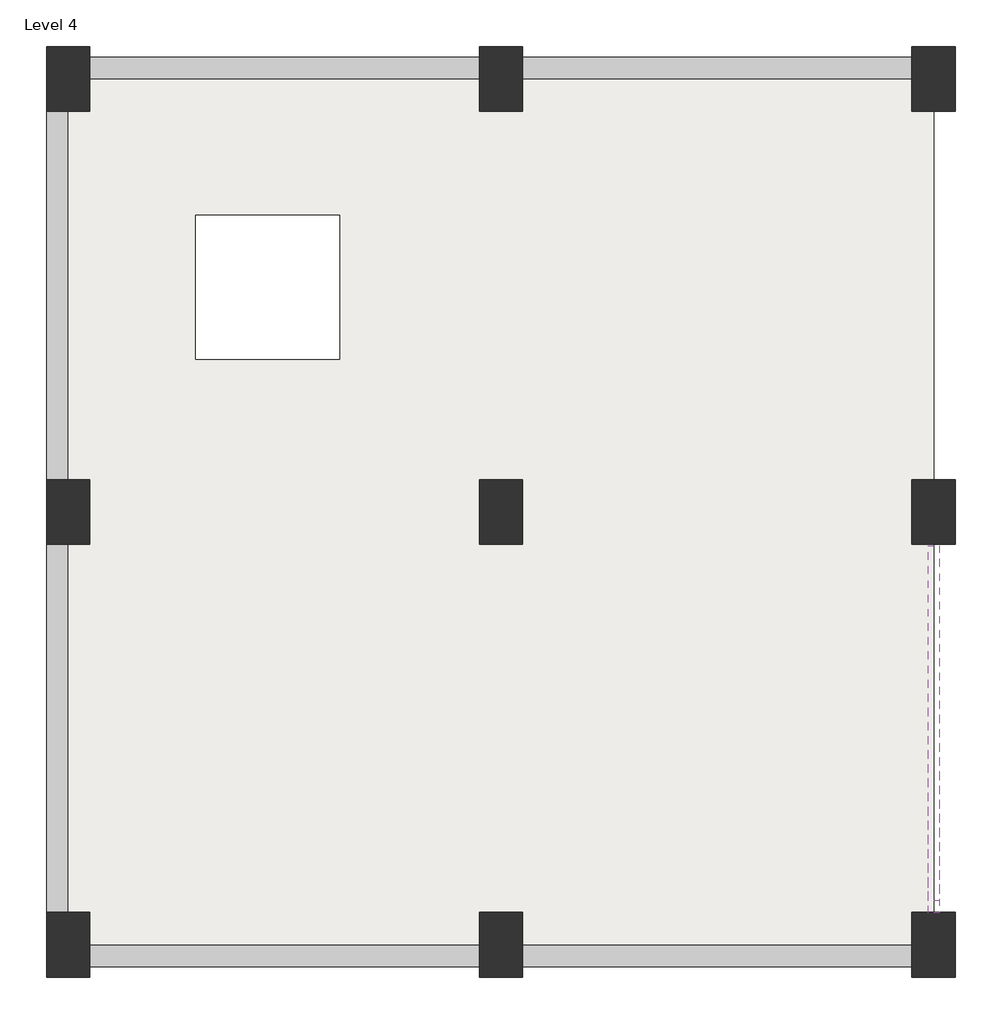
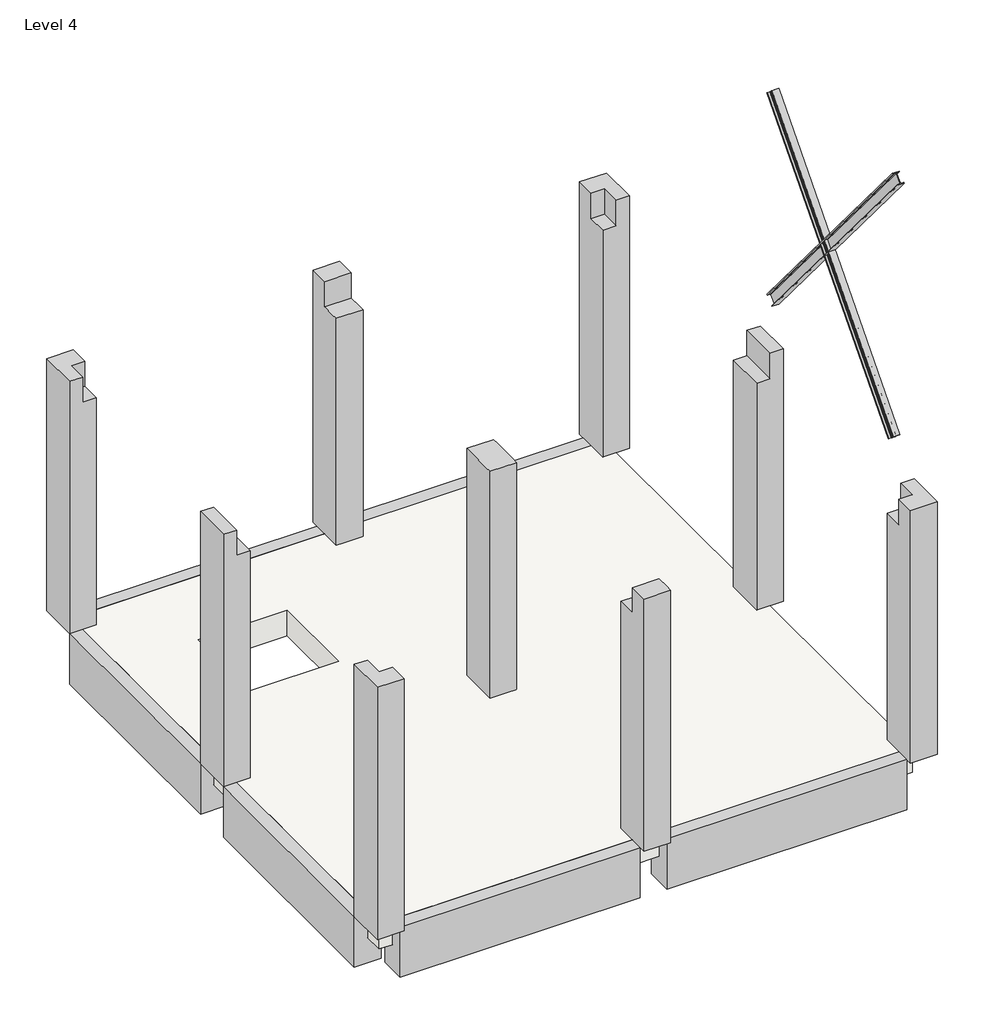
# One storey: 9 columns, 4 beams, 2 members, 2 slabs.
"""IFC4 building model written with IfcOpenShell, lengths in millimetres."""

from ifc_helpers import new_model, si_unit, frame, origin, place, context, project, spatial, polyline, outline, extrude, faceted_brep, transform, mapped, element, save
from components import ub_universal_beams_ub127x76x13_5289bed7, ub_universal_beams_ub127x76x13_b97c8348

model = new_model("IFC4")

# Units and contexts
model_context = context("Model", 3, world=origin())
ifc_project = project(units=[si_unit("LENGTHUNIT", "METRE", prefix="MILLI")], contexts=[model_context])

# Site, building, storey
site = spatial("IfcSite", under=ifc_project)
building = spatial("IfcBuilding", under=site)
storey = spatial("IfcBuildingStorey", under=building, Name="Level 4", Elevation=9000.0)

# Beams
placement = place(None, origin())
element("IfcBeam", 1, ObjectType="Concrete-Rectangular Beam : 300 x 600mm", at=placement, inside=storey, context=model_context, shape_type="SweptSolid", body=[
    extrude(outline(polyline([(526.3372902, 8400.0), (226.3372902, 8400.0), (226.3372902, 8700.0), (376.3372902, 8700.0), (376.3372902, 9000.0), (526.3372902, 9000.0), (526.3372902, 8400.0)])), frame((2068.7595868, 0.0, 0.0), z_axis=(1.0, 0.0, 0.0), x_axis=(0.0, 1.0, 0.0)), (0.0, 0.0, 1.0), 2700.0),
    extrude(outline(polyline([(526.3372902, 8400.0), (226.3372902, 8400.0), (226.3372902, 8700.0), (376.3372902, 8700.0), (376.3372902, 9000.0), (526.3372902, 9000.0), (526.3372902, 8400.0)])), frame((-931.2404132, 0.0, 0.0), z_axis=(1.0, 0.0, 0.0), x_axis=(0.0, 1.0, 0.0)), (0.0, 0.0, 1.0), 2700.0),
])
element("IfcBeam", 2, ObjectType="Concrete-Rectangular Beam : 300 x 600mm", at=placement, inside=storey, context=model_context, shape_type="SweptSolid", body=[
    extrude(outline(polyline([(-5773.6627098, 8400.0), (-5773.6627098, 9000.0), (-5623.6627098, 9000.0), (-5623.6627098, 8700.0), (-5473.6627098, 8700.0), (-5473.6627098, 8400.0), (-5773.6627098, 8400.0)])), frame((2068.7595868, 0.0, 0.0), z_axis=(1.0, 0.0, 0.0), x_axis=(0.0, 1.0, 0.0)), (0.0, 0.0, 1.0), 2700.0),
    extrude(outline(polyline([(-5773.6627098, 8400.0), (-5773.6627098, 9000.0), (-5623.6627098, 9000.0), (-5623.6627098, 8700.0), (-5473.6627098, 8700.0), (-5473.6627098, 8400.0), (-5773.6627098, 8400.0)])), frame((-931.2404132, 0.0, 0.0), z_axis=(1.0, 0.0, 0.0), x_axis=(0.0, 1.0, 0.0)), (0.0, 0.0, 1.0), 2700.0),
])
element("IfcBeam", 3, ObjectType="Concrete-Rectangular Beam : 300 x 600mm", at=placement, inside=storey, context=model_context, shape_type="SweptSolid", body=[
    extrude(outline(polyline([(9000.0, -1231.2404132), (8400.0, -1231.2404132), (8400.0, -931.2404132), (8700.0, -931.2404132), (8700.0, -1081.2404132), (9000.0, -1081.2404132), (9000.0, -1231.2404132)])), frame((0.0, -5398.6627098, 0.0), z_axis=(0.0, 1.0, 0.0), x_axis=(0.0, 0.0, 1.0)), (0.0, 0.0, 1.0), 2550.0),
    extrude(outline(polyline([(9000.0, -1231.2404132), (8400.0, -1231.2404132), (8400.0, -931.2404132), (8700.0, -931.2404132), (8700.0, -1081.2404132), (9000.0, -1081.2404132), (9000.0, -1231.2404132)])), frame((0.0, -2398.6627098, 0.0), z_axis=(0.0, 1.0, 0.0), x_axis=(0.0, 0.0, 1.0)), (0.0, 0.0, 1.0), 2550.0),
])
element("IfcBeam", 4, ObjectType="Concrete-Rectangular Beam : 300 x 600mm", at=placement, inside=storey, context=model_context, shape_type="SweptSolid", body=[
    extrude(outline(polyline([(2068.7595868, -2773.6627098), (2068.7595868, -2473.6627098), (4768.7595868, -2473.6627098), (4768.7595868, -2773.6627098), (2068.7595868, -2773.6627098)])), frame((0.0, 0.0, 8400.0), z_axis=(0.0, 0.0, 1.0), x_axis=(1.0, 0.0, 0.0)), (0.0, 0.0, 1.0), 300.0),
    extrude(outline(polyline([(-931.2404132, -2773.6627098), (-931.2404132, -2473.6627098), (1768.7595868, -2473.6627098), (1768.7595868, -2773.6627098), (-931.2404132, -2773.6627098)])), frame((0.0, 0.0, 8400.0), z_axis=(0.0, 0.0, 1.0), x_axis=(1.0, 0.0, 0.0)), (0.0, 0.0, 1.0), 300.0),
])

# Columns
element("IfcColumn", 5, ObjectType="Concrete-Rectangular-Column : 300 x 450mm", at=placement, inside=storey, context=model_context, shape_type="Brep", body=[
    faceted_brep([(-1231.2404132, -5848.6627098, 12000.0), (-931.2404132, -5848.6627098, 12000.0), (-931.2404132, -5623.6627098, 12000.0), (-1081.2404132, -5623.6627098, 12000.0), (-1081.2404132, -5398.6627098, 12000.0), (-1231.2404132, -5398.6627098, 12000.0), (-1231.2404132, -5848.6627098, 9000.0), (-1231.2404132, -5398.6627098, 9000.0), (-931.2404132, -5398.6627098, 9000.0), (-931.2404132, -5848.6627098, 9000.0), (-931.2404132, -5398.6627098, 11700.0), (-931.2404132, -5623.6627098, 11700.0), (-1081.2404132, -5398.6627098, 11700.0), (-1081.2404132, -5623.6627098, 11700.0)], [[[0, 1, 2, 3, 4, 5]], [[6, 7, 8, 9]], [[1, 0, 6, 9]], [[9, 8, 10, 11, 2, 1]], [[8, 7, 5, 4, 12, 10]], [[0, 5, 7, 6]], [[12, 13, 11, 10]], [[13, 3, 2, 11]], [[3, 13, 12, 4]]]),
])
element("IfcColumn", 6, ObjectType="Concrete-Rectangular-Column : 300 x 450mm", at=placement, inside=storey, context=model_context, shape_type="Brep", body=[
    faceted_brep([(1768.7595868, -5848.6627098, 12000.0), (2068.7595868, -5848.6627098, 12000.0), (2068.7595868, -5773.6627098, 12000.0), (2068.7595868, -5623.6627098, 12000.0), (1768.7595868, -5623.6627098, 12000.0), (1768.7595868, -5773.6627098, 12000.0), (1768.7595868, -5848.6627098, 9000.0), (1768.7595868, -5398.6627098, 9000.0), (2068.7595868, -5398.6627098, 9000.0), (2068.7595868, -5848.6627098, 9000.0), (2068.7595868, -5398.6627098, 11700.0), (2068.7595868, -5473.6627098, 11700.0), (2068.7595868, -5623.6627098, 11700.0), (1768.7595868, -5398.6627098, 11700.0), (1768.7595868, -5623.6627098, 11700.0), (1768.7595868, -5473.6627098, 11700.0)], [[[0, 1, 2, 3, 4, 5]], [[6, 7, 8, 9]], [[1, 0, 6, 9]], [[9, 8, 10, 11, 12, 3, 2, 1]], [[8, 7, 13, 10]], [[7, 6, 0, 5, 4, 14, 15, 13]], [[14, 12, 11, 10, 13, 15]], [[12, 14, 4, 3]]]),
])
element("IfcColumn", 7, ObjectType="Concrete-Rectangular-Column : 300 x 450mm", at=placement, inside=storey, context=model_context, shape_type="Brep", body=[
    faceted_brep([(4768.7595868, -5848.6627098, 12000.0), (5068.7595868, -5848.6627098, 12000.0), (5068.7595868, -5398.6627098, 12000.0), (4918.7595868, -5398.6627098, 12000.0), (4918.7595868, -5623.6627098, 12000.0), (4768.7595868, -5623.6627098, 12000.0), (4768.7595868, -5848.6627098, 9000.0), (4768.7595868, -5398.6627098, 9000.0), (5068.7595868, -5398.6627098, 9000.0), (5068.7595868, -5848.6627098, 9000.0), (4768.7595868, -5398.6627098, 11700.0), (4918.7595868, -5398.6627098, 11700.0), (4768.7595868, -5623.6627098, 11700.0), (4918.7595868, -5623.6627098, 11700.0)], [[[0, 1, 2, 3, 4, 5]], [[6, 7, 8, 9]], [[1, 0, 6, 9]], [[2, 1, 9, 8]], [[8, 7, 10, 11, 3, 2]], [[7, 6, 0, 5, 12, 10]], [[12, 13, 11, 10]], [[13, 4, 3, 11]], [[4, 13, 12, 5]]]),
])
element("IfcColumn", 8, ObjectType="Concrete-Rectangular-Column : 300 x 450mm", at=placement, inside=storey, context=model_context, shape_type="Brep", body=[
    faceted_brep([(-1231.2404132, -2398.6627098, 12000.0), (-1231.2404132, -2848.6627098, 12000.0), (-1081.2404132, -2848.6627098, 12000.0), (-1081.2404132, -2398.6627098, 12000.0), (-1231.2404132, -2848.6627098, 9000.0), (-1231.2404132, -2398.6627098, 9000.0), (-931.2404132, -2398.6627098, 9000.0), (-931.2404132, -2848.6627098, 9000.0), (-931.2404132, -2848.6627098, 11400.0), (-931.2404132, -2848.6627098, 11700.0), (-1081.2404132, -2848.6627098, 11700.0), (-1231.2404132, -2848.6627098, 11400.0), (-931.2404132, -2398.6627098, 11400.0), (-931.2404132, -2398.6627098, 11700.0), (-1231.2404132, -2398.6627098, 11400.0), (-1081.2404132, -2398.6627098, 11700.0)], [[[0, 1, 2, 3]], [[4, 5, 6, 7]], [[4, 7, 8, 9, 10, 2, 1, 11]], [[7, 6, 12, 13, 9, 8]], [[6, 5, 14, 0, 3, 15, 13, 12]], [[1, 0, 14, 5, 4, 11]], [[15, 10, 9, 13]], [[10, 15, 3, 2]]]),
])
element("IfcColumn", 9, ObjectType="Concrete-Rectangular-Column : 300 x 450mm", at=placement, inside=storey, context=model_context, shape_type="Brep", body=[
    faceted_brep([(1768.7595868, -2848.6627098, 9000.0), (1768.7595868, -2398.6627098, 9000.0), (2068.7595868, -2398.6627098, 9000.0), (2068.7595868, -2848.6627098, 9000.0), (2068.7595868, -2848.6627098, 11400.0), (2068.7595868, -2848.6627098, 11700.0), (1768.7595868, -2848.6627098, 11700.0), (1768.7595868, -2848.6627098, 11400.0), (2068.7595868, -2398.6627098, 11400.0), (2068.7595868, -2398.6627098, 11700.0), (2068.7595868, -2473.6627098, 11700.0), (2068.7595868, -2773.6627098, 11700.0), (1768.7595868, -2398.6627098, 11400.0), (1768.7595868, -2398.6627098, 11700.0), (1768.7595868, -2773.6627098, 11700.0), (1768.7595868, -2473.6627098, 11700.0)], [[[0, 1, 2, 3]], [[0, 3, 4, 5, 6, 7]], [[3, 2, 8, 9, 10, 11, 5, 4]], [[2, 1, 12, 13, 9, 8]], [[1, 0, 7, 6, 14, 15, 13, 12]], [[6, 5, 11, 10, 9, 13, 15, 14]]]),
])
element("IfcColumn", 10, ObjectType="Concrete-Rectangular-Column : 300 x 450mm", at=placement, inside=storey, context=model_context, shape_type="Brep", body=[
    faceted_brep([(5068.7595868, -2848.6627098, 12000.0), (5068.7595868, -2398.6627098, 12000.0), (4918.7595868, -2398.6627098, 12000.0), (4918.7595868, -2848.6627098, 12000.0), (4768.7595868, -2848.6627098, 9000.0), (4768.7595868, -2398.6627098, 9000.0), (5068.7595868, -2398.6627098, 9000.0), (5068.7595868, -2848.6627098, 9000.0), (5068.7595868, -2848.6627098, 11400.0), (4918.7595868, -2848.6627098, 11700.0), (4768.7595868, -2848.6627098, 11700.0), (4768.7595868, -2848.6627098, 11400.0), (5068.7595868, -2398.6627098, 11400.0), (4768.7595868, -2398.6627098, 11400.0), (4768.7595868, -2398.6627098, 11700.0), (4918.7595868, -2398.6627098, 11700.0)], [[[0, 1, 2, 3]], [[4, 5, 6, 7]], [[4, 7, 8, 0, 3, 9, 10, 11]], [[1, 0, 8, 7, 6, 12]], [[6, 5, 13, 14, 15, 2, 1, 12]], [[5, 4, 11, 10, 14, 13]], [[9, 15, 14, 10]], [[15, 9, 3, 2]]]),
])
element("IfcColumn", 11, ObjectType="Concrete-Rectangular-Column : 300 x 450mm", at=placement, inside=storey, context=model_context, shape_type="Brep", body=[
    faceted_brep([(-931.2404132, 601.3372902, 12000.0), (-1231.2404132, 601.3372902, 12000.0), (-1231.2404132, 151.3372902, 12000.0), (-1081.2404132, 151.3372902, 12000.0), (-1081.2404132, 376.3372902, 12000.0), (-931.2404132, 376.3372902, 12000.0), (-1231.2404132, 151.3372902, 9000.0), (-1231.2404132, 601.3372902, 9000.0), (-931.2404132, 601.3372902, 9000.0), (-931.2404132, 151.3372902, 9000.0), (-931.2404132, 151.3372902, 11700.0), (-1081.2404132, 151.3372902, 11700.0), (-931.2404132, 376.3372902, 11700.0), (-1081.2404132, 376.3372902, 11700.0)], [[[0, 1, 2, 3, 4, 5]], [[6, 7, 8, 9]], [[6, 9, 10, 11, 3, 2]], [[9, 8, 0, 5, 12, 10]], [[1, 0, 8, 7]], [[2, 1, 7, 6]], [[12, 13, 11, 10]], [[13, 4, 3, 11]], [[4, 13, 12, 5]]]),
])
element("IfcColumn", 12, ObjectType="Concrete-Rectangular-Column : 300 x 450mm", at=placement, inside=storey, context=model_context, shape_type="Brep", body=[
    faceted_brep([(2068.7595868, 601.3372902, 12000.0), (1768.7595868, 601.3372902, 12000.0), (1768.7595868, 526.3372902, 12000.0), (1768.7595868, 376.3372902, 12000.0), (2068.7595868, 376.3372902, 12000.0), (2068.7595868, 526.3372902, 12000.0), (1768.7595868, 151.3372902, 9000.0), (1768.7595868, 601.3372902, 9000.0), (2068.7595868, 601.3372902, 9000.0), (2068.7595868, 151.3372902, 9000.0), (2068.7595868, 151.3372902, 11700.0), (1768.7595868, 151.3372902, 11700.0), (2068.7595868, 376.3372902, 11700.0), (2068.7595868, 226.3372902, 11700.0), (1768.7595868, 226.3372902, 11700.0), (1768.7595868, 376.3372902, 11700.0)], [[[0, 1, 2, 3, 4, 5]], [[6, 7, 8, 9]], [[6, 9, 10, 11]], [[9, 8, 0, 5, 4, 12, 13, 10]], [[1, 0, 8, 7]], [[7, 6, 11, 14, 15, 3, 2, 1]], [[12, 15, 14, 11, 10, 13]], [[15, 12, 4, 3]]]),
])
element("IfcColumn", 13, ObjectType="Concrete-Rectangular-Column : 300 x 450mm", at=placement, inside=storey, context=model_context, shape_type="Brep", body=[
    faceted_brep([(5068.7595868, 151.3372902, 12000.0), (5068.7595868, 601.3372902, 12000.0), (4768.7595868, 601.3372902, 12000.0), (4768.7595868, 376.3372902, 12000.0), (4918.7595868, 376.3372902, 12000.0), (4918.7595868, 151.3372902, 12000.0), (4768.7595868, 151.3372902, 9000.0), (4768.7595868, 601.3372902, 9000.0), (5068.7595868, 601.3372902, 9000.0), (5068.7595868, 151.3372902, 9000.0), (4918.7595868, 151.3372902, 11700.0), (4768.7595868, 151.3372902, 11700.0), (4768.7595868, 376.3372902, 11700.0), (4918.7595868, 376.3372902, 11700.0)], [[[0, 1, 2, 3, 4, 5]], [[6, 7, 8, 9]], [[6, 9, 0, 5, 10, 11]], [[1, 0, 9, 8]], [[2, 1, 8, 7]], [[7, 6, 11, 12, 3, 2]], [[13, 12, 11, 10]], [[4, 13, 10, 5]], [[13, 4, 3, 12]]]),
])

# Members
ub_universal_beams_ub127x76x13_shape = ub_universal_beams_ub127x76x13_5289bed7(model_context)
element("IfcMember", 14, ObjectType="UB-Universal Beams : UB127x76x13", at=placement, inside=storey, context=model_context, shape_type="MappedRepresentation", body=[
    mapped(ub_universal_beams_ub127x76x13_shape, transform((4918.7595868, -3987.3365723, 13970.50801), x_axis=(0.0, 0.6417839133356917, -0.7668855250841063), y_axis=(-1.0, 0.0, 0.0), z_axis=(0.0, 0.7668855250841063, 0.6417839133356917))),
])
ub_universal_beams_ub127x76x13_2_shape = ub_universal_beams_ub127x76x13_b97c8348(model_context)
element("IfcMember", 15, ObjectType="UB-Universal Beams : UB127x76x13", at=placement, inside=storey, context=model_context, shape_type="MappedRepresentation", body=[
    mapped(ub_universal_beams_ub127x76x13_2_shape, transform((4918.7595868, -3946.516498, 13976.6450694), x_axis=(0.0, -0.6614316775001309, -0.7500054239799623), y_axis=(1.0, 0.0, 0.0), z_axis=(0.0, -0.7500054239799623, 0.6614316775001309))),
])

# Slabs
element("IfcSlab", 16, ObjectType="Generic 300mm", at=placement, inside=storey, context=model_context, shape_type="Brep", body=[
    faceted_brep([(4918.7595868, 376.3372902, 8700.0), (4918.7595868, 151.3372902, 8700.0), (4918.7595868, -2398.6627098, 8700.0), (4918.7595868, -2848.6627098, 8700.0), (4918.7595868, -5398.6627098, 8700.0), (4918.7595868, -5623.6627098, 8700.0), (4768.7595868, -5623.6627098, 8700.0), (2068.7595868, -5623.6627098, 8700.0), (1768.7595868, -5623.6627098, 8700.0), (-931.2404132, -5623.6627098, 8700.0), (-1081.2404132, -5623.6627098, 8700.0), (-1081.2404132, -5398.6627098, 8700.0), (-1081.2404132, -2848.6627098, 8700.0), (-1081.2404132, -2398.6627098, 8700.0), (-1081.2404132, 151.3372902, 8700.0), (-1081.2404132, 376.3372902, 8700.0), (-931.2404132, 376.3372902, 8700.0), (1768.7595868, 376.3372902, 8700.0), (2068.7595868, 376.3372902, 8700.0), (4768.7595868, 376.3372902, 8700.0), (-198.5229478, -1566.5574371, 8700.0), (801.4770522, -1566.5574371, 8700.0), (801.4770522, -566.5574371, 8700.0), (-198.5229478, -566.5574371, 8700.0), (4918.7595868, -5623.6627098, 9000.0), (4918.7595868, -5398.6627098, 9000.0), (4918.7595868, -2848.6627098, 9000.0), (4918.7595868, -2398.6627098, 9000.0), (4918.7595868, 151.3372902, 9000.0), (4918.7595868, 376.3372902, 9000.0), (4768.7595868, 376.3372902, 9000.0), (2068.7595868, 376.3372902, 9000.0), (1768.7595868, 376.3372902, 9000.0), (-931.2404132, 376.3372902, 9000.0), (-1081.2404132, 376.3372902, 9000.0), (-1081.2404132, 151.3372902, 9000.0), (-1081.2404132, -2398.6627098, 9000.0), (-1081.2404132, -2848.6627098, 9000.0), (-1081.2404132, -5398.6627098, 9000.0), (-1081.2404132, -5623.6627098, 9000.0), (-931.2404132, -5623.6627098, 9000.0), (1768.7595868, -5623.6627098, 9000.0), (2068.7595868, -5623.6627098, 9000.0), (4768.7595868, -5623.6627098, 9000.0), (801.4770522, -1566.5574371, 9000.0), (-198.5229478, -1566.5574371, 9000.0), (-198.5229478, -566.5574371, 9000.0), (801.4770522, -566.5574371, 9000.0)], [[[0, 1, 2, 3, 4, 5, 6, 7, 8, 9, 10, 11, 12, 13, 14, 15, 16, 17, 18, 19], [20, 21, 22, 23]], [[24, 25, 26, 27, 28, 29, 30, 31, 32, 33, 34, 35, 36, 37, 38, 39, 40, 41, 42, 43], [44, 45, 46, 47]], [[5, 4, 3, 2, 1, 0, 29, 28, 27, 26, 25, 24]], [[10, 9, 8, 7, 6, 5, 24, 43, 42, 41, 40, 39]], [[15, 14, 13, 12, 11, 10, 39, 38, 37, 36, 35, 34]], [[0, 19, 18, 17, 16, 15, 34, 33, 32, 31, 30, 29]], [[20, 45, 44, 21]], [[21, 44, 47, 22]], [[22, 47, 46, 23]], [[45, 20, 23, 46]]]),
])
element("IfcSlab", 17, ObjectType="Generic 300mm", at=placement, inside=storey, context=model_context, shape_type="Brep", body=[
    faceted_brep([(4918.7595868, 376.3372902, 8700.0), (4918.7595868, 151.3372902, 8700.0), (4918.7595868, -2398.6627098, 8700.0), (4918.7595868, -2848.6627098, 8700.0), (4918.7595868, -5398.6627098, 8700.0), (4918.7595868, -5623.6627098, 8700.0), (4768.7595868, -5623.6627098, 8700.0), (2068.7595868, -5623.6627098, 8700.0), (1768.7595868, -5623.6627098, 8700.0), (-931.2404132, -5623.6627098, 8700.0), (-1081.2404132, -5623.6627098, 8700.0), (-1081.2404132, -5398.6627098, 8700.0), (-1081.2404132, -2848.6627098, 8700.0), (-1081.2404132, -2398.6627098, 8700.0), (-1081.2404132, 151.3372902, 8700.0), (-1081.2404132, 376.3372902, 8700.0), (-931.2404132, 376.3372902, 8700.0), (1768.7595868, 376.3372902, 8700.0), (2068.7595868, 376.3372902, 8700.0), (4768.7595868, 376.3372902, 8700.0), (-198.5229478, -1566.5574371, 8700.0), (801.4770522, -1566.5574371, 8700.0), (801.4770522, -566.5574371, 8700.0), (-198.5229478, -566.5574371, 8700.0), (4918.7595868, -5623.6627098, 9000.0), (4918.7595868, -5398.6627098, 9000.0), (4918.7595868, -2848.6627098, 9000.0), (4918.7595868, -2398.6627098, 9000.0), (4918.7595868, 151.3372902, 9000.0), (4918.7595868, 376.3372902, 9000.0), (4768.7595868, 376.3372902, 9000.0), (2068.7595868, 376.3372902, 9000.0), (1768.7595868, 376.3372902, 9000.0), (-931.2404132, 376.3372902, 9000.0), (-1081.2404132, 376.3372902, 9000.0), (-1081.2404132, 151.3372902, 9000.0), (-1081.2404132, -2398.6627098, 9000.0), (-1081.2404132, -2848.6627098, 9000.0), (-1081.2404132, -5398.6627098, 9000.0), (-1081.2404132, -5623.6627098, 9000.0), (-931.2404132, -5623.6627098, 9000.0), (1768.7595868, -5623.6627098, 9000.0), (2068.7595868, -5623.6627098, 9000.0), (4768.7595868, -5623.6627098, 9000.0), (801.4770522, -1566.5574371, 9000.0), (-198.5229478, -1566.5574371, 9000.0), (-198.5229478, -566.5574371, 9000.0), (801.4770522, -566.5574371, 9000.0)], [[[0, 1, 2, 3, 4, 5, 6, 7, 8, 9, 10, 11, 12, 13, 14, 15, 16, 17, 18, 19], [20, 21, 22, 23]], [[24, 25, 26, 27, 28, 29, 30, 31, 32, 33, 34, 35, 36, 37, 38, 39, 40, 41, 42, 43], [44, 45, 46, 47]], [[5, 4, 3, 2, 1, 0, 29, 28, 27, 26, 25, 24]], [[10, 9, 8, 7, 6, 5, 24, 43, 42, 41, 40, 39]], [[15, 14, 13, 12, 11, 10, 39, 38, 37, 36, 35, 34]], [[0, 19, 18, 17, 16, 15, 34, 33, 32, 31, 30, 29]], [[20, 45, 44, 21]], [[21, 44, 47, 22]], [[22, 47, 46, 23]], [[45, 20, 23, 46]]]),
])

save(model, "model.ifc")

# Revit data of these elements
# Type "Concrete-Rectangular Beam : 300 x 600mm"
#   Length [instance default] = 1.524 m
#   b = 0.3 m
#   h = 0.6 m
#   Structural Material [instance default] = Concrete, Cast-in-Place gray
#   Assembly Code = ""
# Type "Concrete-Rectangular-Column : 300 x 450mm"
#   b = 0.3 m
#   h = 0.45 m
#   Structural Material [instance default] = Concrete, Cast-in-Place gray
# Type "UB-Universal Beams : UB127x76x13"
#   Section Name Key = "UB127X76X13"
#   Width = 7.6 cm
#   Web Thickness = 0.4 cm
#   Web Fillet = 0.76 cm
#   Warping Constant = 2000.0 cm⁶
#   Torsional Moment of Inertia = 2.85 cm⁴
#   Section Area = 16.5 cm²
#   Plastic Modulus weak axis = 22.6 cm³
#   Plastic Modulus strong axis = 84.2 cm³
#   Nominal Weight = 13.00 kgf/m
#   Moment of Inertia weak axis = 55.70 cm⁴
#   Moment of Inertia strong axis = 473.00 cm⁴
#   Height = 12.7 cm
#   Flange Thickness = 0.76 cm
#   Elastic Modulus weak axis = 14.7 cm³
#   Elastic Modulus strong axis = 74.6 cm³
#   Centroid Vertical = 6.35 cm
#   Centroid Horizontal = 3.8 cm
#   Bolt Spacing = 4.0 cm
#   Length [instance default] = 1.5 m
#   Structural Material [instance default] = Metal - Steel 43-275
#   Type Comments = ""
#   Assembly Code = ""
# Type "Generic 300mm"
#   Function = 0
#   Layers, outside or top first: 0.3 m no material (function 1)
# Elements 1, 2, 3, 4 (IfcBeam, "Concrete-Rectangular Beam : 300 x 600mm")
#   Structural Material = Concrete, Cast-in-Place gray
#   Phase Created = New Construction
#   Materials on its faces: "Concrete, Cast-in-Place gray"
# Elements 5, 6, 7, 8, 9, 10, 11, 12, 13 (IfcColumn, "Concrete-Rectangular-Column : 300 x 450mm")
#   Structural Material = Concrete, Cast-in-Place gray
#   Phase Created = New Construction
#   Materials on its faces: "Concrete, Cast-in-Place gray"
# Elements 14, 15 (IfcMember, "UB-Universal Beams : UB127x76x13")
#   Structural Material = Metal - Steel 43-275
#   Phase Created = New Construction
#   Materials on its faces: "Metal - Steel 43-275"
# Elements 16, 17 (IfcSlab, "Generic 300mm")
#   Height Offset From Level = 0 m
#   built-in parameter 1001954 = 1
#   Phase Created = New Construction
#   Materials on its faces: "Default Floor"
# Materials
#   "Concrete, Cast-in-Place gray": class "Concrete", colour RGB 192 192 192, transparency 0, Description = "Cast-in-place concrete", Cost = 0
#   "Metal - Steel 43-275": class "Metal", colour RGB 247 247 247, transparency 0, Cost = 0
#   "Default Floor": colour RGB 127 127 127, transparency 0, Cost = 0
